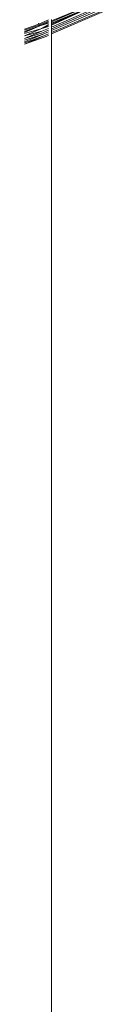
# Model space of a CAD drawing. Units: inches. Extents: x 64 to 1167, y 117 to 939.
# Tile 41 of 56: x 1130.649 to 1130.735, y 498.834 to 499.913. Entities that reach past the tile are written whole.
import ezdxf

# ---------------------------------------------------------------- set-up
doc = ezdxf.new("R2010")
doc.units = ezdxf.units.IN
doc.header["$MEASUREMENT"] = 0
doc.layers.add('A-FLOR-FIXT', color=8, linetype='Continuous', lineweight=18)

msp = doc.modelspace()

# ---------------------------------------------------------------- linework, layer by layer
at = {"layer": 'A-FLOR-FIXT'}
for p, q in [((1130.6784, 499.9108), (1130.7302, 499.9332)), ((1130.6784, 499.912), (1130.7302, 499.9332)), ((1130.6784, 499.9084), (1130.7311, 499.9312)), ((1130.6784, 499.9096), (1130.7311, 499.9312)), ((1130.6784, 499.9073), (1130.7311, 499.9312)), ((1130.6784, 499.9051), (1130.7324, 499.9284)), ((1130.6784, 499.9031), (1130.7332, 499.9268)), ((1130.6784, 499.9013), (1130.7339, 499.9253)), ((1130.6784, 499.8991), (1130.7348, 499.9235)), ((1130.6784, 499.8976), (1130.7354, 499.9222)), ((1130.6646, 499.9085), (1130.6751, 499.9131)), ((1130.665, 499.9074), (1130.6751, 499.9118)), ((1130.6784, 499.9133), (1130.6784, 499.9108)), ((1130.6487, 499.9028), (1130.6646, 499.9085)), ((1130.6487, 499.9016), (1130.665, 499.9074)), ((1130.6487, 499.8992), (1130.6655, 499.9064)), ((1130.6487, 499.9004), (1130.6655, 499.9064)), ((1130.6487, 499.8957), (1130.6667, 499.9033)), ((1130.6487, 499.898), (1130.6667, 499.9033)), ((1130.6642, 499.9096), (1130.6646, 499.9085)), ((1130.6646, 499.9085), (1130.665, 499.9074)), ((1130.665, 499.9074), (1130.6655, 499.9064)), ((1130.6655, 499.9064), (1130.6751, 499.9106)), ((1130.6655, 499.9064), (1130.6751, 499.9093)), ((1130.6667, 499.9033), (1130.6751, 499.9081)), ((1130.6667, 499.9033), (1130.6751, 499.907)), ((1130.6667, 499.9033), (1130.6751, 499.9058)), ((1130.6678, 499.9005), (1130.6751, 499.9036)), ((1130.6685, 499.8988), (1130.6751, 499.9016)), ((1130.6784, 499.9108), (1130.6784, 499.9084)), ((1130.6784, 499.9084), (1130.6784, 499.9051)), ((1130.6784, 499.9051), (1130.6784, 499.9031)), ((1130.6784, 499.9031), (1130.6784, 499.9013)), ((1130.6784, 499.9013), (1130.6784, 499.8991)), ((1130.6487, 499.8926), (1130.6678, 499.9005)), ((1130.6487, 499.8957), (1130.6678, 499.9005)), ((1130.6487, 499.8926), (1130.6685, 499.8988)), ((1130.6487, 499.8908), (1130.6691, 499.8973)), ((1130.6487, 499.8891), (1130.6691, 499.8973)), ((1130.6487, 499.8878), (1130.6698, 499.8954)), ((1130.6487, 499.8863), (1130.6698, 499.8954)), ((1130.6487, 499.8863), (1130.6703, 499.8941)), ((1130.6691, 499.8973), (1130.6751, 499.8999)), ((1130.6698, 499.8954), (1130.6751, 499.8977)), ((1130.6703, 499.8941), (1130.6751, 499.8961)), ((1130.6784, 499.8991), (1130.6784, 499.8976)), ((1130.6784, 499.8976), (1130.6784, 490.2192))]:
    msp.add_line(p, q, dxfattribs=at)

doc.saveas('drawing.dxf')
